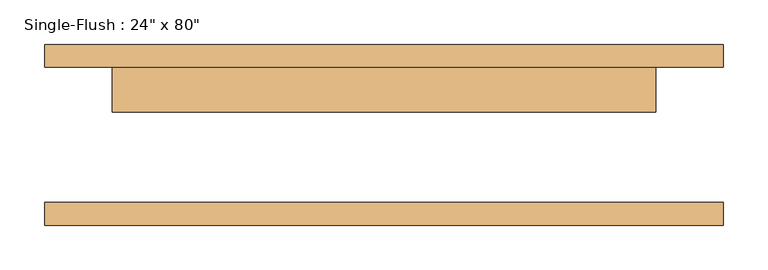
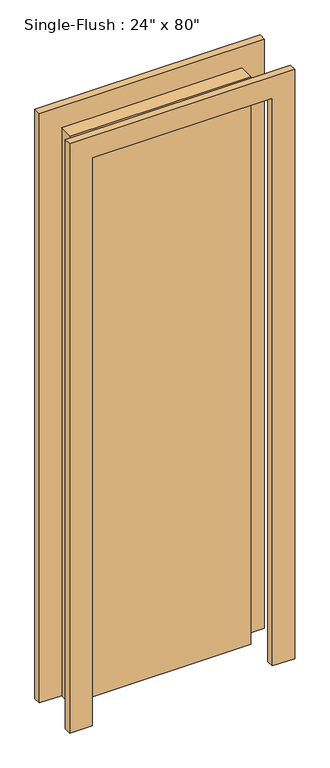
"""IFC4 building model written with IfcOpenShell, lengths in millimetres: door geometry."""

from ifc_helpers import new_model, si_unit, frame, origin, origin_with_axes, place, context, project, spatial, polyline, outline, extrude, source, transform, mapped, element, save


def door_58dae0ba(model_context):
    return source(origin(), model_context, "Body", "SweptSolid", [
        extrude(outline(polyline([(2108.2, -381.0), (0.0, -381.0), (0.0, -304.8), (2032.0, -304.8), (2032.0, 304.8), (0.0, 304.8), (0.0, 381.0), (2108.2, 381.0), (2108.2, -381.0)])), frame((0.0, 76.2, 0.0), z_axis=(0.0, 1.0, 0.0), x_axis=(0.0, 0.0, 1.0)), (0.0, 0.0, 1.0), 25.4),
        extrude(outline(polyline([(2108.2, 381.0), (2108.2, -381.0), (0.0, -381.0), (0.0, -304.8), (2032.0, -304.8), (2032.0, 304.8), (0.0, 304.8), (0.0, 381.0), (2108.2, 381.0)])), frame((0.0, -101.6, 0.0), z_axis=(0.0, 1.0, 0.0), x_axis=(0.0, 0.0, 1.0)), (0.0, 0.0, 1.0), 25.4),
        extrude(outline(polyline([(304.8, 25.4), (-304.8, 25.4), (-304.8, 76.2), (304.8, 76.2), (304.8, 25.4)])), origin_with_axes(), (0.0, 0.0, 1.0), 2032.0),
    ])


if __name__ == "__main__":
    model = new_model("IFC4")
    model_context = context("Model", 3, world=origin())
    ifc_project = project(units=[si_unit("LENGTHUNIT", "METRE", prefix="MILLI")], contexts=[model_context])
    site = spatial("IfcSite", under=ifc_project)
    building = spatial("IfcBuilding", under=site)
    placement = place(None, origin())
    door_shape = door_58dae0ba(model_context)
    element("IfcDoor", 1, ObjectType="Single-Flush : 24\" x 80\"", at=placement, inside=building, context=model_context, shape_type="MappedRepresentation", body=[
        mapped(door_shape, transform((0.0, 0.0, 0.0), x_axis=(1.0, 0.0, 0.0), y_axis=(0.0, 1.0, 0.0), z_axis=(0.0, 0.0, 1.0))),
    ])
    save(model, "model.ifc")

# Revit data of these elements
# Type "Single-Flush : 24\" x 80\""
#   Type Mark = "5"
#   Construction Type Id = "MDOOR"
#   Assembly Code = "C1020"
#   Analytic Construction = "Metal"
#   Thickness = 0' - 2"
#   Heat Transfer Coefficient (U) = 0.651978 BTU/(h·ft²·°F)
#   Height = 6' - 8"
#   Trim Projection Ext = 0' - 1"
#   Trim Projection Int = 0' - 1"
#   Trim Width = 0' - 3"
#   Width = 2' - 0"
#   Define Thermal Properties by = 1
#   Door Material = Door - Panel
#   Frame Material = Door - Frame
#   Visual Light Transmittance = 0
#   Solar Heat Gain Coefficient = 0
#   Function = (empty or 0)
#   Wall Closure = (empty or 0)
# Element 1 (IfcDoor, "Single-Flush : 24\" x 80\"")
#   Materials on its faces: "Door - Frame", "Door - Panel"
# Materials
#   "Door - Panel": class "Wood", colour RGB 210 159 95, transparency 0
#   "Door - Frame": colour RGB 118 70 51, transparency 0
